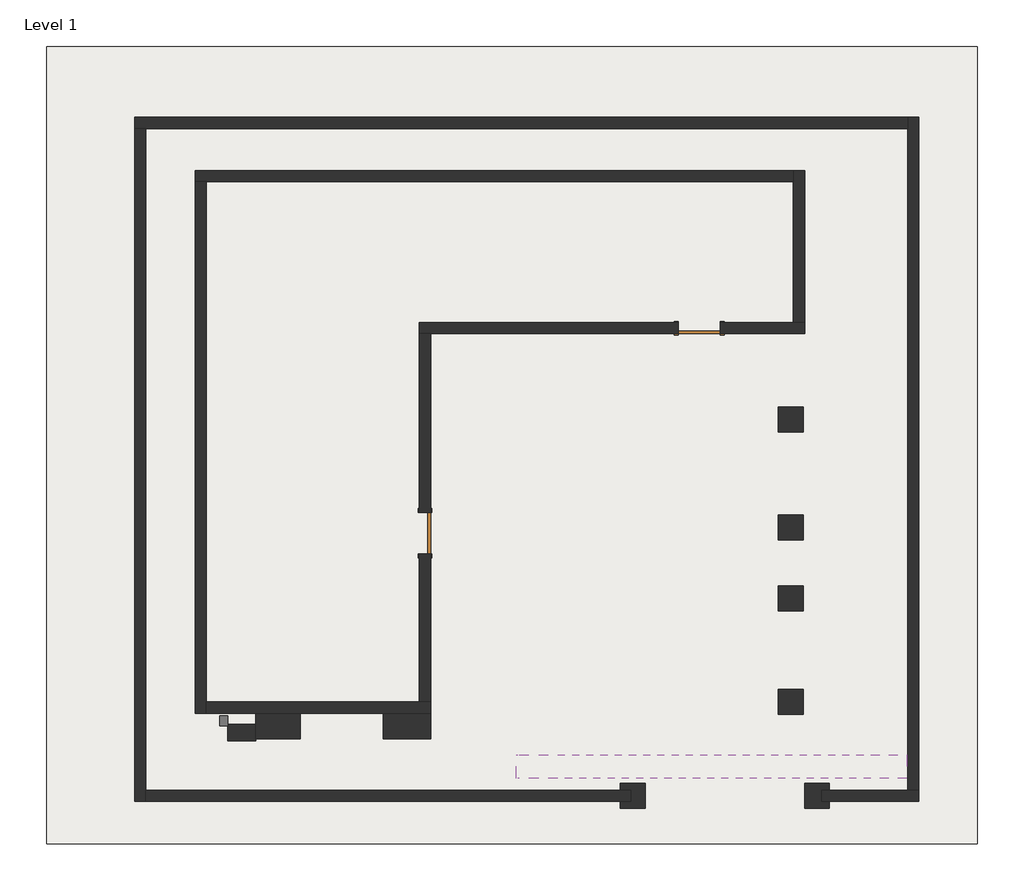
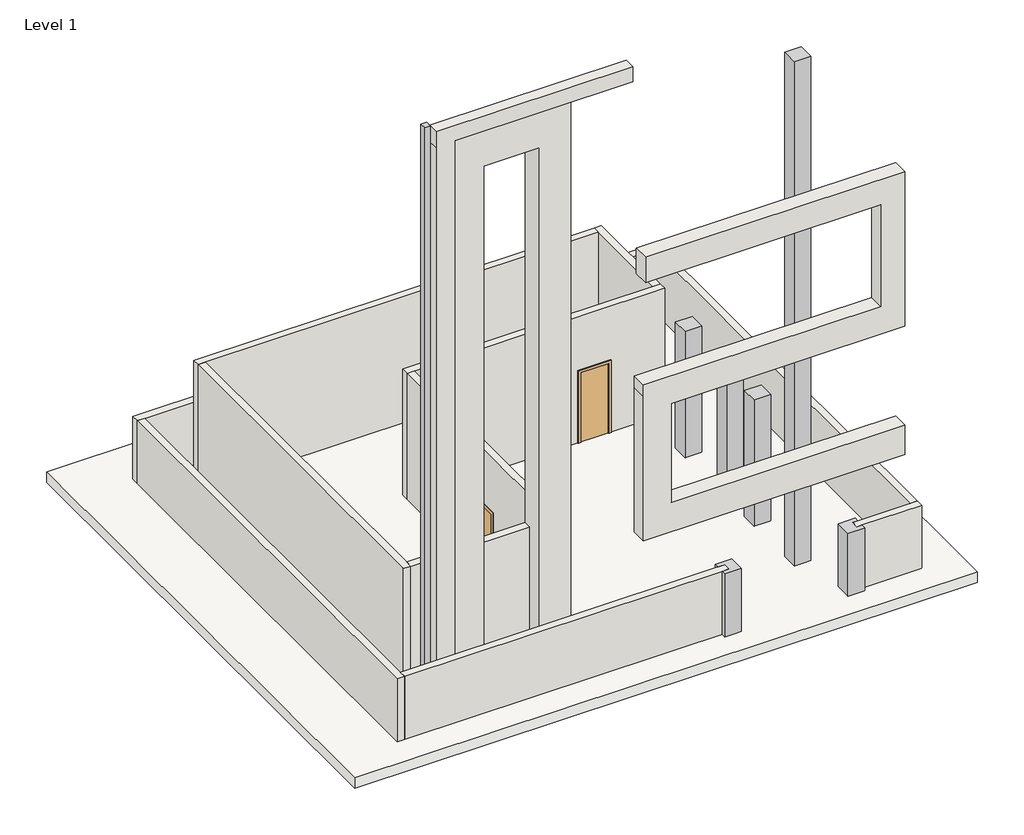
# One storey: 13 walls, 6 columns, 2 doors, 1 proxy, 1 slab.
"""IFC4 building model written with IfcOpenShell, lengths in millimetres."""

from ifc_helpers import new_model, si_unit, frame, origin, origin_with_axes, place, context, project, spatial, polyline, outline, extrude, faceted_brep, transform, mapped, element, save
from components import column_59a13550, door_fadea3f2, walls_1_walls_1_82da7aad, walls_2_walls_2_8cca178c, walls_3_walls_3_bbde4dad

model = new_model("IFC4")

# Units and contexts
model_context = context("Model", 3, world=origin())
ifc_project = project(units=[si_unit("LENGTHUNIT", "METRE", prefix="MILLI")], contexts=[model_context])

# Site, building, storey
site = spatial("IfcSite", under=ifc_project)
building = spatial("IfcBuilding", under=site)
storey = spatial("IfcBuildingStorey", under=building, Name="Level 1", Elevation=0.0)

# Proxy
placement = place(None, origin())
element("IfcBuildingElementProxy", 1, Name="Reveal", ObjectType="Reveal", at=placement, inside=storey, context=model_context, shape_type="SweptSolid", body=[
    extrude(outline(polyline([(-10501.0871298, 910.8559817), (-10501.0871298, 1093.7359817), (-10348.6871298, 1093.7359817), (-10348.6871298, 910.8559817), (-10501.0871298, 910.8559817)])), origin_with_axes(), (0.0, 0.0, 1.0), 16422.5278597),
])

# Columns
element("IfcColumn", 2, ObjectType="Rectangular Column : 18\" x 18\"", at=placement, inside=storey, context=model_context, shape_type="SweptSolid", body=[
    extrude(outline(polyline([(198.6628702, 4776.7359817), (198.6628702, 4319.5359817), (-258.5371298, 4319.5359817), (-258.5371298, 4776.7359817), (198.6628702, 4776.7359817)])), origin_with_axes(), (0.0, 0.0, 1.0), 3657.6),
])
element("IfcColumn", 3, ObjectType="Rectangular Column : 18\" x 18\"", at=placement, inside=storey, context=model_context, shape_type="SweptSolid", body=[
    extrude(outline(polyline([(198.6628702, 6757.9359817), (198.6628702, 6300.7359817), (-258.5371298, 6300.7359817), (-258.5371298, 6757.9359817), (198.6628702, 6757.9359817)])), origin_with_axes(), (0.0, 0.0, 1.0), 3657.6),
])
element("IfcColumn", 4, ObjectType="Rectangular Column : 18\" x 18\"", at=placement, inside=storey, context=model_context, shape_type="SweptSolid", body=[
    extrude(outline(polyline([(198.6628702, 3481.3359817), (198.6628702, 3024.1359817), (-258.5371298, 3024.1359817), (-258.5371298, 3481.3359817), (198.6628702, 3481.3359817)])), origin_with_axes(), (0.0, 0.0, 1.0), 3657.6),
])
element("IfcColumn", 5, ObjectType="Rectangular Column : 18\" x 18\"", at=placement, inside=storey, context=model_context, shape_type="SweptSolid", body=[
    extrude(outline(polyline([(-2696.9371298, -143.9149728), (-2696.9371298, -601.1149728), (-3154.1371298, -601.1149728), (-3154.1371298, -474.1149728), (-2964.696544, -474.1149728), (-2964.696544, -270.9149728), (-3154.1371298, -270.9149728), (-3154.1371298, -143.9149728), (-2696.9371298, -143.9149728)])), origin_with_axes(), (0.0, 0.0, 1.0), 1828.8),
])
element("IfcColumn", 6, ObjectType="Rectangular Column : 18\" x 18\"", at=placement, inside=storey, context=model_context, shape_type="SweptSolid", body=[
    extrude(outline(polyline([(681.2628702, -601.1149728), (224.0628702, -601.1149728), (224.0628702, -143.9149728), (681.2628702, -143.9149728), (681.2628702, -270.9149728), (540.503456, -270.9149728), (540.503456, -474.1149728), (681.2628702, -474.1149728), (681.2628702, -601.1149728)])), origin_with_axes(), (0.0, 0.0, 1.0), 1828.8),
])
column_shape = column_59a13550(model_context)
element("IfcColumn", 7, ObjectType="Rectangular Column : 18\" x 18\"", at=placement, inside=storey, context=model_context, shape_type="MappedRepresentation", body=[
    mapped(column_shape, transform((-29.9371298, 1347.7359817, 0.0), x_axis=(1.0, 0.0, 0.0), y_axis=(0.0, 1.0, 0.0), z_axis=(0.0, 0.0, 1.0))),
])

# Doors
door_shape = door_fadea3f2(model_context)
element("IfcDoor", 8, ObjectType="Single-Flush : 30\" x 80\"", at=placement, inside=storey, context=model_context, shape_type="MappedRepresentation", body=[
    mapped(door_shape, transform((-1706.3371298, 8205.7359817, 0.0), x_axis=(-1.0, 0.0, 0.0), y_axis=(0.0, -1.0, 0.0), z_axis=(0.0, 0.0, 1.0))),
])
element("IfcDoor", 9, ObjectType="Single-Flush : 30\" x 80\"", at=placement, inside=storey, context=model_context, shape_type="MappedRepresentation", body=[
    mapped(door_shape, transform((-6735.5371298, 4446.5359817, 0.0), x_axis=(0.0, -1.0, 0.0), y_axis=(1.0, 0.0, 0.0), z_axis=(0.0, 0.0, 1.0))),
])

# Slab
element("IfcSlab", 10, ObjectType="Generic - 12\"", at=placement, inside=storey, context=model_context, shape_type="SweptSolid", body=[
    extrude(outline(polyline([(3394.4882391, 13374.4419215), (3394.4882391, -1255.9580785), (-13674.3117609, -1255.9580785), (-13674.3117609, 13374.4419215), (3394.4882391, 13374.4419215)])), frame((0.0, 0.0, -304.8), z_axis=(0.0, 0.0, 1.0), x_axis=(1.0, 0.0, 0.0)), (0.0, 0.0, 1.0), 304.8),
])

# Walls
element("IfcWall", 11, ObjectType="Generic - 8\"", at=placement, inside=storey, context=model_context, shape_type="Brep", body=[
    faceted_brep([(-10951.9371298, 10898.1359817, 0.0), (-10748.7371298, 10898.1359817, 0.0), (20.8628702, 10898.1359817, 0.0), (20.8628702, 10898.1359817, 3657.6), (-10748.7371298, 10898.1359817, 3657.6), (-10951.9371298, 10898.1359817, 3657.6), (-10951.9371298, 11101.3359817, 0.0), (-10951.9371298, 11101.3359817, 3657.6), (20.8628702, 11101.3359817, 3657.6), (20.8628702, 11101.3359817, 0.0)], [[[0, 1, 2, 3, 4, 5]], [[6, 7, 8, 9]], [[2, 1, 0, 6, 9]], [[0, 5, 7, 6]], [[3, 2, 9, 8]], [[5, 4, 3, 8, 7]]]),
])
element("IfcWall", 12, ObjectType="Generic - 8\"", at=placement, inside=storey, context=model_context, shape_type="Brep", body=[
    faceted_brep([(-10748.7371298, 1144.5359817, 0.0), (-10748.7371298, 1347.7359817, 0.0), (-10748.7371298, 10898.1359817, 0.0), (-10748.7371298, 10898.1359817, 3657.6), (-10748.7371298, 1347.7359817, 3657.6), (-10748.7371298, 1144.5359817, 3657.6), (-10951.9371298, 1144.5359817, 0.0), (-10951.9371298, 1144.5359817, 3657.6), (-10951.9371298, 10898.1359817, 3657.6), (-10951.9371298, 10898.1359817, 0.0)], [[[0, 1, 2, 3, 4, 5]], [[6, 7, 8, 9]], [[2, 1, 0, 6, 9]], [[0, 5, 7, 6]], [[3, 2, 9, 8]], [[5, 4, 3, 8, 7]]]),
])
element("IfcWall", 13, ObjectType="Generic - 8\"", at=placement, inside=storey, context=model_context, shape_type="Brep", body=[
    faceted_brep([(-6633.9371298, 1347.7359817, 0.0), (-6837.1371298, 1347.7359817, 0.0), (-10748.7371298, 1347.7359817, 0.0), (-10748.7371298, 1347.7359817, 3657.6), (-6837.1371298, 1347.7359817, 3657.6), (-6633.9371298, 1347.7359817, 3657.6), (-6633.9371298, 1144.5359817, 0.0), (-6633.9371298, 1144.5359817, 3657.6), (-10748.7371298, 1144.5359817, 3657.6), (-10748.7371298, 1144.5359817, 0.0)], [[[0, 1, 2, 3, 4, 5]], [[6, 7, 8, 9]], [[2, 1, 0, 6, 9]], [[3, 2, 9, 8]], [[5, 4, 3, 8, 7]], [[0, 5, 7, 6]]]),
])
element("IfcWall", 14, ObjectType="Generic - 8\"", at=placement, inside=storey, context=model_context, shape_type="Brep", body=[
    faceted_brep([(20.8628702, 11101.3359817, 0.0), (20.8628702, 10898.1359817, 0.0), (20.8628702, 8307.3359817, 0.0), (20.8628702, 8307.3359817, 3657.6), (20.8628702, 10898.1359817, 3657.6), (20.8628702, 11101.3359817, 3657.6), (224.0628702, 11101.3359817, 0.0), (224.0628702, 11101.3359817, 3657.6), (224.0628702, 8307.3359817, 3657.6), (224.0628702, 8307.3359817, 0.0)], [[[0, 1, 2, 3, 4, 5]], [[6, 7, 8, 9]], [[2, 1, 0, 6, 9]], [[0, 5, 7, 6]], [[5, 4, 3, 8, 7]], [[3, 2, 9, 8]]]),
])
element("IfcWall", 15, ObjectType="Generic - 8\"", at=placement, inside=storey, context=model_context, shape_type="Brep", body=[
    faceted_brep([(-2087.3371298, 8307.3359817, 2032.0), (-2087.3371298, 8307.3359817, 0.0), (-6837.1371298, 8307.3359817, 0.0), (-6837.1371298, 8307.3359817, 3657.6), (20.8628702, 8307.3359817, 3657.6), (224.0628702, 8307.3359817, 3657.6), (224.0628702, 8307.3359817, 0.0), (20.8628702, 8307.3359817, 0.0), (-1325.3371298, 8307.3359817, 0.0), (-1325.3371298, 8307.3359817, 2032.0), (-6837.1371298, 8104.1359817, 0.0), (-6633.9371298, 8104.1359817, 0.0), (-2087.3371298, 8104.1359817, 0.0), (-2087.3371298, 8104.1359817, 2032.0), (-1325.3371298, 8104.1359817, 2032.0), (-1325.3371298, 8104.1359817, 0.0), (224.0628702, 8104.1359817, 0.0), (224.0628702, 8104.1359817, 3657.6), (-6633.9371298, 8104.1359817, 3657.6), (-6837.1371298, 8104.1359817, 3657.6)], [[[0, 1, 2, 3, 4, 5, 6, 7, 8, 9]], [[10, 11, 12, 13, 14, 15, 16, 17, 18, 19]], [[2, 1, 12, 11, 10]], [[8, 7, 6, 16, 15]], [[5, 4, 3, 19, 18, 17]], [[3, 2, 10, 19]], [[6, 5, 17, 16]], [[13, 12, 1, 0]], [[14, 13, 0, 9]], [[15, 14, 9, 8]]]),
])
element("IfcWall", 16, ObjectType="Generic - 8\"", at=placement, inside=storey, context=model_context, shape_type="SweptSolid", body=[
    extrude(outline(polyline([(4065.5359817, 2032.0), (4065.5359817, 0.0), (1347.7359817, 0.0), (1347.7359817, 3657.6), (8104.1359817, 3657.6), (8104.1359817, 0.0), (4827.5359817, 0.0), (4827.5359817, 2032.0), (4065.5359817, 2032.0)])), frame((-6837.1371298, 0.0, 0.0), z_axis=(1.0, 0.0, 0.0), x_axis=(0.0, 1.0, 0.0)), (0.0, 0.0, 1.0), 203.2),
])
element("IfcWall", 17, ObjectType="Generic - 8\"", at=placement, inside=storey, context=model_context, shape_type="Brep", body=[
    faceted_brep([(-12057.896544, 11870.2850272, 0.0), (-11854.696544, 11870.2850272, 0.0), (2115.303456, 11870.2850272, 0.0), (2115.303456, 11870.2850272, 1828.8), (-11854.696544, 11870.2850272, 1828.8), (-12057.896544, 11870.2850272, 1828.8), (-12057.896544, 12073.4850272, 0.0), (-12057.896544, 12073.4850272, 1828.8), (2115.303456, 12073.4850272, 1828.8), (2115.303456, 12073.4850272, 0.0)], [[[0, 1, 2, 3, 4, 5]], [[6, 7, 8, 9]], [[2, 1, 0, 6, 9]], [[5, 4, 3, 8, 7]], [[0, 5, 7, 6]], [[3, 2, 9, 8]]]),
])
element("IfcWall", 18, ObjectType="Generic - 8\"", at=placement, inside=storey, context=model_context, shape_type="Brep", body=[
    faceted_brep([(-11854.696544, -474.1149728, 0.0), (-11854.696544, -270.9149728, 0.0), (-11854.696544, 11870.2850272, 0.0), (-11854.696544, 11870.2850272, 1828.8), (-11854.696544, -270.9149728, 1828.8), (-11854.696544, -474.1149728, 1828.8), (-12057.896544, -474.1149728, 0.0), (-12057.896544, -474.1149728, 1828.8), (-12057.896544, 11870.2850272, 1828.8), (-12057.896544, 11870.2850272, 0.0)], [[[0, 1, 2, 3, 4, 5]], [[6, 7, 8, 9]], [[2, 1, 0, 6, 9]], [[5, 4, 3, 8, 7]], [[0, 5, 7, 6]], [[3, 2, 9, 8]]]),
])
element("IfcWall", 19, ObjectType="Generic - 8\"", at=placement, inside=storey, context=model_context, shape_type="Brep", body=[
    faceted_brep([(2318.503456, -270.9149728, 0.0), (2115.303456, -270.9149728, 0.0), (681.2628702, -270.9149728, 0.0), (540.503456, -270.9149728, 0.0), (540.503456, -270.9149728, 1828.8), (681.2628702, -270.9149728, 1828.8), (2115.303456, -270.9149728, 1828.8), (2318.503456, -270.9149728, 1828.8), (2318.503456, -474.1149728, 0.0), (2318.503456, -474.1149728, 1828.8), (681.2628702, -474.1149728, 1828.8), (540.503456, -474.1149728, 1828.8), (540.503456, -474.1149728, 0.0), (681.2628702, -474.1149728, 0.0)], [[[0, 1, 2, 3, 4, 5, 6, 7]], [[8, 9, 10, 11, 12, 13]], [[0, 7, 9, 8]], [[3, 2, 1, 0, 8, 13, 12]], [[4, 3, 12, 11]], [[7, 6, 5, 4, 11, 10, 9]]]),
    faceted_brep([(-11854.696544, -270.9149728, 1828.8), (-3154.1371298, -270.9149728, 1828.8), (-2964.696544, -270.9149728, 1828.8), (-2964.696544, -270.9149728, 0.0), (-3154.1371298, -270.9149728, 0.0), (-11854.696544, -270.9149728, 0.0), (-11854.696544, -474.1149728, 1828.8), (-11854.696544, -474.1149728, 0.0), (-3154.1371298, -474.1149728, 0.0), (-2964.696544, -474.1149728, 0.0), (-2964.696544, -474.1149728, 1828.8), (-3154.1371298, -474.1149728, 1828.8)], [[[0, 1, 2, 3, 4, 5]], [[6, 7, 8, 9, 10, 11]], [[0, 5, 7, 6]], [[2, 1, 0, 6, 11, 10]], [[3, 2, 10, 9]], [[5, 4, 3, 9, 8, 7]]]),
])
element("IfcWall", 20, ObjectType="Generic - 8\"", at=placement, inside=storey, context=model_context, shape_type="Brep", body=[
    faceted_brep([(2115.303456, 12073.4850272, 0.0), (2115.303456, 11870.2850272, 0.0), (2115.303456, -270.9149728, 0.0), (2115.303456, -270.9149728, 1828.8), (2115.303456, 11870.2850272, 1828.8), (2115.303456, 12073.4850272, 1828.8), (2318.503456, 12073.4850272, 0.0), (2318.503456, 12073.4850272, 1828.8), (2318.503456, -270.9149728, 1828.8), (2318.503456, -270.9149728, 0.0)], [[[0, 1, 2, 3, 4, 5]], [[6, 7, 8, 9]], [[2, 1, 0, 6, 9]], [[5, 4, 3, 8, 7]], [[0, 5, 7, 6]], [[3, 2, 9, 8]]]),
])
walls_1_walls_1_shape = walls_1_walls_1_82da7aad(model_context)
element("IfcWall", 21, ObjectType="Walls 1 : Walls 1", at=placement, inside=storey, context=model_context, shape_type="MappedRepresentation", body=[
    mapped(walls_1_walls_1_shape, transform((0.0, 0.0, 0.0), x_axis=(1.0, 0.0, 0.0), y_axis=(0.0, 1.0, 0.0), z_axis=(0.0, 0.0, 1.0))),
])
walls_2_walls_2_shape = walls_2_walls_2_8cca178c(model_context)
element("IfcWall", 22, ObjectType="Walls 2 : Walls 2", at=placement, inside=storey, context=model_context, shape_type="MappedRepresentation", body=[
    mapped(walls_2_walls_2_shape, transform((0.0, 0.0, 0.0), x_axis=(1.0, 0.0, 0.0), y_axis=(0.0, 1.0, 0.0), z_axis=(0.0, 0.0, 1.0))),
])
walls_3_walls_3_shape = walls_3_walls_3_bbde4dad(model_context)
element("IfcWall", 23, ObjectType="Walls 3 : Walls 3", at=placement, inside=storey, context=model_context, shape_type="MappedRepresentation", body=[
    mapped(walls_3_walls_3_shape, transform((0.0, 0.0, 0.0), x_axis=(1.0, 0.0, 0.0), y_axis=(0.0, 1.0, 0.0), z_axis=(0.0, 0.0, 1.0))),
])

save(model, "model.ifc")

# Revit data of these elements
# Type "Rectangular Column : 18\" x 18\""
#   Assembly Code = "B1010200"
#   Depth = 1' - 6"
#   Offset Base = 0' - 0"
#   Offset Top = 0' - 0"
#   Width = 1' - 6"
#   Material = none
# Type "Single-Flush : 30\" x 80\""
#   Type Mark = "5"
#   Construction Type Id = "MDOOR"
#   Assembly Code = "C1020"
#   Analytic Construction = "Metal"
#   Thickness = 0' - 2"
#   Heat Transfer Coefficient (U) = 0.651978 BTU/(h·ft²·°F)
#   Height = 6' - 8"
#   Trim Projection Ext = 0' - 1"
#   Trim Projection Int = 0' - 1"
#   Trim Width = 0' - 3"
#   Width = 2' - 6"
#   Define Thermal Properties by = 1
#   Door Material = Door - Panel
#   Frame Material = Door - Frame
#   Visual Light Transmittance = 0
#   Solar Heat Gain Coefficient = 0
#   Function = (empty or 0)
#   Wall Closure = (empty or 0)
# Type "Generic - 12\""
#   Assembly Code = "B1010"
#   Function = 0
#   Layers, outside or top first: 1' - 0" no material (function 1)
# Type "Generic - 8\""
#   Assembly Code = "B2010"
#   Layers, outside or top first: 0' - 8" no material (function 1)
# Elements 2, 3, 5, 6 (IfcColumn, "Rectangular Column : 18\" x 18\"")
#   Phase Created = New Construction
#   Materials on its faces: "Default Wall"
# Elements 4, 7 (IfcColumn, "Rectangular Column : 18\" x 18\"")
#   Phase Created = New Construction
# Elements 8, 9 (IfcDoor, "Single-Flush : 30\" x 80\"")
#   Phase Created = New Construction
#   Materials on its faces: "Door - Frame", "Door - Panel"
# Element 10 (IfcSlab, "Generic - 12\"")
#   Height Offset From Level = 0' - 0"
#   Phase Created = New Construction
#   Materials on its faces: "Default Floor"
# Elements 11, 12, 13, 14, 15, 16 (IfcWall, "Generic - 8\"")
#   Top Offset = 0' - 0"
#   Base Offset = 0' - 0"
#   Unconnected Height = 12' - 0"
#   wall height = 12' - 0"
#   Phase Created = New Construction
#   Base Constraint = Level 1
#   Materials on its faces: "Default Wall"
# Elements 17, 18, 19, 20 (IfcWall, "Generic - 8\"")
#   Top Offset = 0' - 0"
#   Base Offset = 0' - 0"
#   Unconnected Height = 6' - 0"
#   wall height = 6' - 0"
#   Phase Created = New Construction
#   Base Constraint = Level 1
#   Materials on its faces: "Default Wall"
# Element 21 (IfcWall, "Walls 1 : Walls 1")
#   Phase Created = New Construction
#   Materials on its faces: "Default Wall"
# Element 22 (IfcWall, "Walls 2 : Walls 2")
#   Phase Created = New Construction
#   Materials on its faces: "Default Wall"
# Element 23 (IfcWall, "Walls 3 : Walls 3")
#   Phase Created = New Construction
#   Materials on its faces: "Default Wall"
# Materials
#   "Door - Panel": class "Wood", colour RGB 210 159 95, transparency 0
#   "Door - Frame": colour RGB 118 70 51, transparency 0
#   "Default Wall": colour RGB 128 128 128, transparency 0
#   "Default Floor": colour RGB 128 128 128, transparency 0
